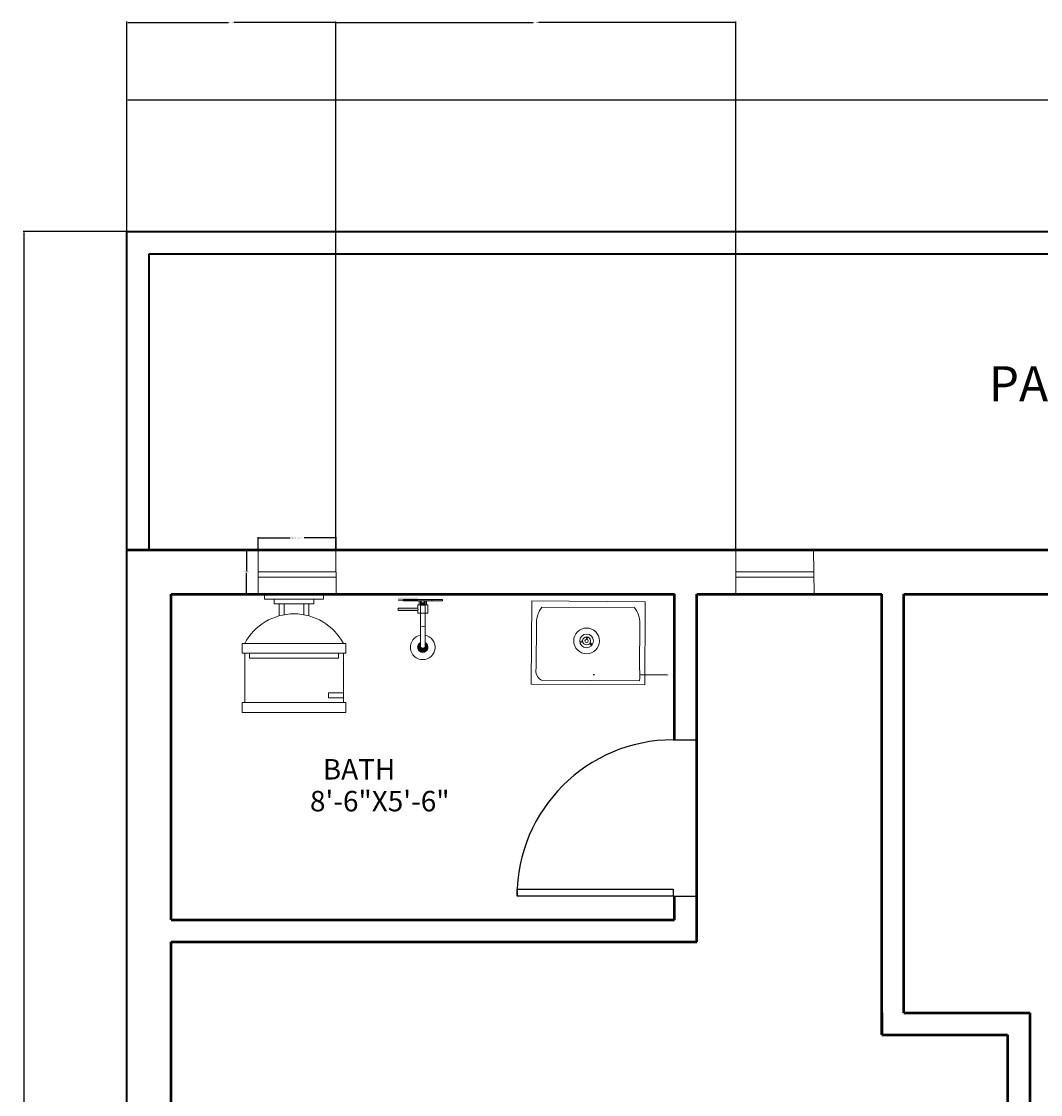
# Model space of a CAD drawing. Units: inches. Extents: x -44 to 461, y -6 to 860.
# Tile 3 of 7: x -23 to 184, y 642 to 860. Entities that reach past the tile are written whole.
import ezdxf

# ---------------------------------------------------------------- set-up
doc = ezdxf.new("R2010")
doc.units = ezdxf.units.IN
doc.header["$MEASUREMENT"] = 0
for name, color, linetype, lineweight in [('A-ANNO-DIMS', 2, 'Continuous', 18), ('A-AREA-IDEN', 7, 'Continuous', 18), ('A-DOOR', 4, 'Continuous', 25), ('C-PROP', 7, 'Continuous', 35), ('PLUMBING FIXTURES', 8, 'Continuous', 18), ('walls', 8, 'Continuous', 50), ('windows', 171, 'Continuous', 18)]:
    doc.layers.add(name, color=color, linetype=linetype, lineweight=lineweight)
doc.styles.get("Standard").update_dxf_attribs({"font": 'arial.ttf'})
doc.dimstyles.get("Standard").update_dxf_attribs({"dimtxt": 0.18, "dimasz": 0.18, "dimexe": 0.18, "dimexo": 0.0625, "dimgap": 0.09, "dimtad": 0, "dimtih": 1, "dimtoh": 1, "dimdec": 4, "dimzin": 0, "dimdsep": 46, "dimtxsty": 'Standard', "dimcen": 0.09, "dimadec": 0, "dimazin": 0, "dimtfac": 1, "dimtdec": 4, "dimtofl": 0, "dimtmove": 0, "dimatfit": 3, "dimfxl": 1, "dimtolj": 1, "dimtzin": 0, "dimarcsym": 0})

# ---------------------------------------------------------------- blocks, each defined once
blk = doc.blocks.new('*U10')
for p, q in [((-10, 22), (-10, 12)), ((10, 12), (10, 22)), ((-10, 21), (-7, 21)), ((-7, 20), (-10, 20)), ((-7, 21), (-7, 20)), ((10.5, 12), (-10.5, 12)), ((-10.5, 10), (-10.5, 12)), ((9, 13), (-9, 13)), ((-9, 13), (-9, 12)), ((9, 12), (9, 13)), ((10.5, 12), (10.5, 10)), ((10.5, 10), (-10.5, 10)), ((-3, 4.4065), (-3, 2)), ((3, 2), (3, 4.4065)), ((-2, 2), (-2, 4.1658)), ((2, 4.1658), (2, 2)), ((4, 2), (-4, 2)), ((-4, 2), (-4, 1)), ((4, 1), (4, 2))]:
    blk.add_line(p, q)
for points in [[(10.5, 22), (10.5, 24), (-10.5, 24), (-10.5, 22)], [(6, 0), (6, 1), (-6, 1), (-6, 0)]]:
    blk.add_lwpolyline(points, close=True)
blk.add_arc((0, 15.3333), 11.3333, 208.0725, 331.9275)
blk = doc.blocks.new('*U12')
for p, q in [((0, 0), (0, -6)), ((40, 0), (40, -6))]:
    blk.add_line(p, q)
blk.add_lwpolyline([(0, 0), (0, 40), (1.75, 40), (1.75, 0)], close=True)
blk.add_arc((0, 0), 40, 0, 90)
blk = doc.blocks.new('*D18')
at = {"layer": 'A-ANNO-DIMS', "color": 0, "lineweight": -2, "transparency": 16777216}
for p, q in [((-1.55, 817.11), (-1.55, 843.94)), ((-1.37, 843.76), (207.84, 843.76)), ((418.27, 843.76), (209.05, 843.76)), ((418.45, 817.11), (418.45, 843.94))]:
    blk.add_line(p, q, dxfattribs=at)
at = {"layer": 'A-ANNO-DIMS', "color": 0, "transparency": 16777216}
for points in [[(-1.37, 843.79), (-1.37, 843.73), (-1.55, 843.76)], [(418.27, 843.79), (418.27, 843.73), (418.45, 843.76)]]:
    blk.add_solid(points, dxfattribs=at)
at = {"layer": 'Defpoints', "color": 0, "transparency": 16777216}
for p in [(418.45, 843.76), (-1.55, 817.05), (418.45, 817.05)]:
    blk.add_point(p, dxfattribs=at)
at = {"layer": 'A-ANNO-DIMS', "color": 0, "transparency": 16777216, "insert": (208.45, 843.76), "char_height": 0.18, "attachment_point": 5}
blk.add_mtext('\\A1;420.0000', dxfattribs=at)
blk = doc.blocks.new('*D19')
at = {"layer": 'A-ANNO-DIMS', "color": 0, "lineweight": -2, "transparency": 16777216}
for p, q in [((-1.62, 817.05), (-22.6, 817.05)), ((-22.42, 816.87), (-22.42, 427.23)), ((-22.42, 37.23), (-22.42, 426.87)), ((-1.62, 37.05), (-22.6, 37.05))]:
    blk.add_line(p, q, dxfattribs=at)
at = {"layer": 'A-ANNO-DIMS', "color": 0, "transparency": 16777216}
for points in [[(-22.45, 816.87), (-22.39, 816.87), (-22.42, 817.05)], [(-22.45, 37.23), (-22.39, 37.23), (-22.42, 37.05)]]:
    blk.add_solid(points, dxfattribs=at)
at = {"layer": 'Defpoints', "color": 0, "transparency": 16777216}
for p in [(-22.42, 817.05), (-1.55, 817.05), (-1.55, 37.05)]:
    blk.add_point(p, dxfattribs=at)
at = {"layer": 'A-ANNO-DIMS', "color": 0, "transparency": 16777216, "insert": (-22.42, 427.05), "char_height": 0.18, "attachment_point": 5}
blk.add_mtext('\\A1;780.0000', dxfattribs=at)
blk = doc.blocks.new('WIN-16IN-FRAME')
for p, q in [((0, 0), (0, 9)), ((0, 9), (15.73, 9)), ((15.73, 9), (15.83, 0)), ((15.78, 4.5), (0, 4.5)), ((0, 0), (0, 3.42)), ((0, 3.42), (15.78, 3.42)), ((0.11, 0), (15.83, 0))]:
    blk.add_line(p, q)
blk = doc.blocks.new('LAV-RECTANGULAR')
for p, q in [((0, 0.15), (0.11, 17)), ((0.11, 17), (23.11, 16.85)), ((20.97, 15.65), (2.16, 15.77)), ((23.1, 15.71), (23, 0)), ((23.11, 16.85), (23.1, 15.71)), ((0.99, 3.35), (1.05, 12.64)), ((21.97, 3.21), (22.03, 12.5)), ((10.4, 8.91), (9.84, 8.81)), ((11.22, 9.73), (11.17, 9.24)), ((11.36, 9.22), (11.4, 9.7)), ((10.52, 8.7), (9.87, 8.58)), ((11.84, 8.39), (12.22, 7.95)), ((11.97, 8.6), (12.36, 8.13)), ((23, 0), (0, 0.15)), ((21.95, 0.84), (2.06, 0.97))]:
    blk.add_line(p, q)
for radius in [2.61, 1.39, 0.816, 0.338]:
    blk.add_circle((11.22, 8.91), radius)
for centre, radius, start, end in [((6.46, 12.5), 5.4, 142.7525, 178.5493), ((16.62, 12.43), 5.4, 0.6949, 36.4918), ((3, 2.82), 2.08, 165.2338, 242.9258), ((12.7, 2.09), 9.33, 352.3124, 6.9318)]:
    blk.add_arc(centre, radius, start, end)
blk = doc.blocks.new('O.H SHOWER-PL')
at = {"layer": 'PLUMBING FIXTURES'}
for points in [[(-1.84, 0), (-1.84, -0.25), (1.84, -0.25), (1.84, 0)], [(0.46, -8.72), (0.46, -9.67, -0.422337), (-0.46, -9.67), (-0.46, -8.72, 4.325472)]]:
    blk.add_hatch(color=256, dxfattribs=at).paths.add_polyline_path(points)
for p, q in [((-1.84, 0), (-1.84, -0.25)), ((1.84, 0), (-1.84, 0)), ((1.84, 0), (1.84, -0.25)), ((1.84, -0.25), (-1.84, -0.25)), ((-0.46, -0.25), (-0.46, -9.67)), ((0.46, -0.25), (0.46, -9.67))]:
    blk.add_line(p, q, dxfattribs=at)
for centre, radius, start, end in [((0, -4.48), 1.03, 243.53, 296.47), ((0, -9.67), 2.5, 100.61, 79.39), ((0, -9.67), 1.05, 116.0349, 63.9652), ((0, -9.22), 0.643, 224.2078, 315.7922)]:
    blk.add_arc(centre, radius, start, end, dxfattribs=at)
blk = doc.blocks.new('DIVERTER-PL')
at = {"layer": 'PLUMBING FIXTURES'}
for points in [[(4, 0), (-4, 0), (-4, -0.25), (4, -0.25)], [(0.38, -1.14), (0.38, -0.7), (-0.37, -0.7), (-0.37, -1.14)], [(1, -1.75, 0.30818), (1, -2.25), (5, -2.25), (5, -1.75)]]:
    blk.add_hatch(color=256, dxfattribs=at).paths.add_polyline_path(points)
for p, q in [((-4, 0), (-4, -0.25)), ((-4, 0), (4, 0)), ((4, 0), (4, -0.25)), ((-4, -0.25), (4, -0.25)), ((-4, -0.25), (4, -0.25)), ((-1, -1.05), (-0.37, -1.05)), ((-1, -1.05), (-1, -2.75)), ((-0.75, -0.25), (-0.75, -1.05)), ((-0.37, -0.7), (0.38, -0.7)), ((-0.37, -0.7), (-0.37, -1.14)), ((-0.37, -1.14), (0.38, -1.14)), ((-0.32, -0.7), (-0.32, -0.25)), ((0.32, -0.7), (0.32, -0.25)), ((0.38, -0.7), (0.38, -1.14)), ((0.38, -1.05), (1, -1.05)), ((0.75, -0.25), (0.75, -1.05)), ((1, -1.05), (1, -1.75)), ((-1, -2.75), (1, -2.75)), ((1, -2.25), (1, -2.75))]:
    blk.add_line(p, q, dxfattribs=at)
at = {"layer": 'PLUMBING FIXTURES', "ltscale": 12}
for p, q in [((1, -1.75), (5, -1.75)), ((5, -2.25), (5, -1.75)), ((1, -2.25), (5, -2.25))]:
    blk.add_line(p, q, dxfattribs=at)
at = {"layer": 'PLUMBING FIXTURES'}
blk.add_arc((1.37, -2), 0.444, 145.7435, 214.2565, dxfattribs=at)
blk = doc.blocks.new('A$C7F153053')
at = {"layer": 'PLUMBING FIXTURES', "xscale": -1, "rotation": 270}
for name in ['DIVERTER-PL', 'O.H SHOWER-PL']:
    blk.add_blockref(name, (12.17, 4), dxfattribs=at)
blk = doc.blocks.new('SHOWER-HEAD-AND-DIVERTER')
for points in [[(4, 12.56, -0.30818), (4, 12.06), (0, 12.06), (0, 12.56)], [(4, 12.56, -0.30818), (4, 12.06), (0, 12.06), (0, 12.56)], [(4, 12.56, -0.30818), (4, 12.06), (0, 12.06), (0, 12.56)], [(4, 12.56, -0.30818), (4, 12.06), (0, 12.06), (0, 12.56)], [(4, 12.56, -0.30818), (4, 12.06), (0, 12.06), (0, 12.56)], [(4, 12.56, -0.30818), (4, 12.06), (0, 12.06), (0, 12.56)], [(4, 12.56, -0.30818), (4, 12.06), (0, 12.06), (0, 12.56)], [(4, 12.56, -0.30818), (4, 12.06), (0, 12.06), (0, 12.56)], [(4, 12.56, -0.30818), (4, 12.06), (0, 12.06), (0, 12.56)], [(4, 12.56, -0.30818), (4, 12.06), (0, 12.06), (0, 12.56)], [(4, 12.56, -0.30818), (4, 12.06), (0, 12.06), (0, 12.56)], [(4, 12.56, -0.30818), (4, 12.06), (0, 12.06), (0, 12.56)], [(4, 12.56, -0.30818), (4, 12.06), (0, 12.06), (0, 12.56)], [(4, 12.56, -0.30818), (4, 12.06), (0, 12.06), (0, 12.56)], [(4, 12.56, -0.30818), (4, 12.06), (0, 12.06), (0, 12.56)], [(4, 12.56, -0.30818), (4, 12.06), (0, 12.06), (0, 12.56)], [(4, 12.56, -0.30818), (4, 12.06), (0, 12.06), (0, 12.56)], [(4, 12.56, -0.30818), (4, 12.06), (0, 12.06), (0, 12.56)], [(4, 12.56, -0.30818), (4, 12.06), (0, 12.06), (0, 12.56)], [(4, 12.56, -0.30818), (4, 12.06), (0, 12.06), (0, 12.56)], [(4, 12.56, -0.30818), (4, 12.06), (0, 12.06), (0, 12.56)], [(4, 12.56, -0.30818), (4, 12.06), (0, 12.06), (0, 12.56)], [(4, 12.56, -0.30818), (4, 12.06), (0, 12.06), (0, 12.56)], [(4, 12.56, -0.30818), (4, 12.06), (0, 12.06), (0, 12.56)], [(4, 12.56, -0.30818), (4, 12.06), (0, 12.06), (0, 12.56)], [(4, 12.56, -0.30818), (4, 12.06), (0, 12.06), (0, 12.56)], [(4, 12.56, -0.30818), (4, 12.06), (0, 12.06), (0, 12.56)], [(4, 12.56, -0.30818), (4, 12.06), (0, 12.06), (0, 12.56)], [(4, 12.56, -0.30818), (4, 12.06), (0, 12.06), (0, 12.56)], [(4, 12.56, -0.30818), (4, 12.06), (0, 12.06), (0, 12.56)], [(4, 12.56, -0.30818), (4, 12.06), (0, 12.06), (0, 12.56)], [(4, 12.56, -0.30818), (4, 12.06), (0, 12.06), (0, 12.56)], [(4, 12.56, -0.30818), (4, 12.06), (0, 12.06), (0, 12.56)], [(4, 12.56, -0.30818), (4, 12.06), (0, 12.06), (0, 12.56)], [(4, 12.56, -0.30818), (4, 12.06), (0, 12.06), (0, 12.56)], [(4, 12.56, -0.30818), (4, 12.06), (0, 12.06), (0, 12.56)], [(4.54, 3.44), (4.54, 2.5, 0.422337), (5.46, 2.5), (5.46, 3.44, -4.325472)], [(4.54, 3.44), (4.54, 2.5, 0.422337), (5.46, 2.5), (5.46, 3.44, -4.325472)], [(4.54, 3.44), (4.54, 2.5, 0.422337), (5.46, 2.5), (5.46, 3.44, -4.325472)], [(4.54, 3.44), (4.54, 2.5, 0.422337), (5.46, 2.5), (5.46, 3.44, -4.325472)], [(4.54, 3.44), (4.54, 2.5, 0.422337), (5.46, 2.5), (5.46, 3.44, -4.325472)], [(4.54, 3.44), (4.54, 2.5, 0.422337), (5.46, 2.5), (5.46, 3.44, -4.325472)], [(4.54, 3.44), (4.54, 2.5, 0.422337), (5.46, 2.5), (5.46, 3.44, -4.325472)], [(4.54, 3.44), (4.54, 2.5, 0.422337), (5.46, 2.5), (5.46, 3.44, -4.325472)], [(4.54, 3.44), (4.54, 2.5, 0.422337), (5.46, 2.5), (5.46, 3.44, -4.325472)], [(4.54, 3.44), (4.54, 2.5, 0.422337), (5.46, 2.5), (5.46, 3.44, -4.325472)], [(4.54, 3.44), (4.54, 2.5, 0.422337), (5.46, 2.5), (5.46, 3.44, -4.325472)], [(4.54, 3.44), (4.54, 2.5, 0.422337), (5.46, 2.5), (5.46, 3.44, -4.325472)], [(4.54, 3.44), (4.54, 2.5, 0.422337), (5.46, 2.5), (5.46, 3.44, -4.325472)], [(4.54, 3.44), (4.54, 2.5, 0.422337), (5.46, 2.5), (5.46, 3.44, -4.325472)], [(4.54, 3.44), (4.54, 2.5, 0.422337), (5.46, 2.5), (5.46, 3.44, -4.325472)], [(4.54, 3.44), (4.54, 2.5, 0.422337), (5.46, 2.5), (5.46, 3.44, -4.325472)], [(4.54, 3.44), (4.54, 2.5, 0.422337), (5.46, 2.5), (5.46, 3.44, -4.325472)], [(4.54, 3.44), (4.54, 2.5, 0.422337), (5.46, 2.5), (5.46, 3.44, -4.325472)], [(4.54, 3.44), (4.54, 2.5, 0.422337), (5.46, 2.5), (5.46, 3.44, -4.325472)], [(4.54, 3.44), (4.54, 2.5, 0.422337), (5.46, 2.5), (5.46, 3.44, -4.325472)], [(4.54, 3.44), (4.54, 2.5, 0.422337), (5.46, 2.5), (5.46, 3.44, -4.325472)], [(4.54, 3.44), (4.54, 2.5, 0.422337), (5.46, 2.5), (5.46, 3.44, -4.325472)], [(4.54, 3.44), (4.54, 2.5, 0.422337), (5.46, 2.5), (5.46, 3.44, -4.325472)], [(4.54, 3.44), (4.54, 2.5, 0.422337), (5.46, 2.5), (5.46, 3.44, -4.325472)], [(4.54, 3.44), (4.54, 2.5, 0.422337), (5.46, 2.5), (5.46, 3.44, -4.325472)], [(4.54, 3.44), (4.54, 2.5, 0.422337), (5.46, 2.5), (5.46, 3.44, -4.325472)], [(4.54, 3.44), (4.54, 2.5, 0.422337), (5.46, 2.5), (5.46, 3.44, -4.325472)], [(4.54, 3.44), (4.54, 2.5, 0.422337), (5.46, 2.5), (5.46, 3.44, -4.325472)], [(4.54, 3.44), (4.54, 2.5, 0.422337), (5.46, 2.5), (5.46, 3.44, -4.325472)], [(4.54, 3.44), (4.54, 2.5, 0.422337), (5.46, 2.5), (5.46, 3.44, -4.325472)], [(4.54, 3.44), (4.54, 2.5, 0.422337), (5.46, 2.5), (5.46, 3.44, -4.325472)], [(4.54, 3.44), (4.54, 2.5, 0.422337), (5.46, 2.5), (5.46, 3.44, -4.325472)], [(4.54, 3.44), (4.54, 2.5, 0.422337), (5.46, 2.5), (5.46, 3.44, -4.325472)], [(4.54, 3.44), (4.54, 2.5, 0.422337), (5.46, 2.5), (5.46, 3.44, -4.325472)], [(4.54, 3.44), (4.54, 2.5, 0.422337), (5.46, 2.5), (5.46, 3.44, -4.325472)], [(4.54, 3.44), (4.54, 2.5, 0.422337), (5.46, 2.5), (5.46, 3.44, -4.325472)], [(4.54, 3.44), (4.54, 2.5, 0.422337), (5.46, 2.5), (5.46, 3.44, -4.325472)], [(4.54, 3.44), (4.54, 2.5, 0.422337), (5.46, 2.5), (5.46, 3.44, -4.325472)]]:
    blk.add_hatch(color=256).paths.add_polyline_path(points)
at = {"ltscale": 12}
blk.add_line((4, 12.06), (0, 12.06), dxfattribs=at)
blk.add_line((4, 12.06), (0, 12.06), dxfattribs=at)
blk.add_line((4, 12.06), (0, 12.06), dxfattribs=at)
blk.add_line((4, 12.06), (0, 12.06), dxfattribs=at)
blk.add_line((4, 12.06), (0, 12.06), dxfattribs=at)
blk.add_line((4, 12.06), (0, 12.06), dxfattribs=at)
blk.add_line((4, 12.06), (0, 12.06), dxfattribs=at)
blk.add_line((4, 12.06), (0, 12.06), dxfattribs=at)
blk.add_line((4, 12.06), (0, 12.06), dxfattribs=at)
blk.add_line((4, 12.06), (0, 12.06), dxfattribs=at)
blk.add_line((4, 12.06), (0, 12.06), dxfattribs=at)
blk.add_line((4, 12.06), (0, 12.06), dxfattribs=at)
blk.add_line((4, 12.06), (0, 12.06), dxfattribs=at)
blk.add_line((4, 12.06), (0, 12.06), dxfattribs=at)
blk.add_line((4, 12.06), (0, 12.06), dxfattribs=at)
blk.add_line((4, 12.06), (0, 12.06), dxfattribs=at)
blk.add_line((4, 12.06), (0, 12.06), dxfattribs=at)
blk.add_line((4, 12.06), (0, 12.06), dxfattribs=at)
blk.add_line((4, 12.06), (0, 12.06), dxfattribs=at)
blk.add_line((4, 12.06), (0, 12.06), dxfattribs=at)
blk.add_line((4, 12.06), (0, 12.06), dxfattribs=at)
blk.add_line((4, 12.06), (0, 12.06), dxfattribs=at)
blk.add_line((4, 12.06), (0, 12.06), dxfattribs=at)
blk.add_line((4, 12.06), (0, 12.06), dxfattribs=at)
blk.add_line((4, 12.06), (0, 12.06), dxfattribs=at)
blk.add_line((4, 12.06), (0, 12.06), dxfattribs=at)
blk.add_line((4, 12.06), (0, 12.06), dxfattribs=at)
blk.add_line((4, 12.06), (0, 12.06), dxfattribs=at)
blk.add_line((4, 12.06), (0, 12.06), dxfattribs=at)
blk.add_line((4, 12.06), (0, 12.06), dxfattribs=at)
blk.add_line((4, 12.06), (0, 12.06), dxfattribs=at)
blk.add_line((4, 12.06), (0, 12.06), dxfattribs=at)
blk.add_line((4, 12.06), (0, 12.06), dxfattribs=at)
blk.add_line((4, 12.06), (0, 12.06), dxfattribs=at)
blk.add_line((4, 12.06), (0, 12.06), dxfattribs=at)
blk.add_line((4, 12.06), (0, 12.06), dxfattribs=at)
blk.add_line((4, 12.06), (0, 12.06), dxfattribs=at)
blk.add_line((4, 12.06), (0, 12.06), dxfattribs=at)
for p, q in [((4.54, 11.92), (4.54, 2.5)), ((4.54, 11.92), (4.54, 2.5)), ((4.54, 11.92), (4.54, 2.5)), ((4.54, 11.92), (4.54, 2.5)), ((4.54, 11.92), (4.54, 2.5)), ((4.54, 11.92), (4.54, 2.5)), ((4.54, 11.92), (4.54, 2.5)), ((4.54, 11.92), (4.54, 2.5)), ((4.54, 11.92), (4.54, 2.5)), ((4.54, 11.92), (4.54, 2.5)), ((4.54, 11.92), (4.54, 2.5)), ((4.54, 11.92), (4.54, 2.5)), ((4.54, 11.92), (4.54, 2.5)), ((4.54, 11.92), (4.54, 2.5)), ((4.54, 11.92), (4.54, 2.5)), ((4.54, 11.92), (4.54, 2.5)), ((4.54, 11.92), (4.54, 2.5)), ((4.54, 11.92), (4.54, 2.5)), ((4.54, 11.92), (4.54, 2.5)), ((4.54, 11.92), (4.54, 2.5)), ((4.54, 11.92), (4.54, 2.5)), ((4.54, 11.92), (4.54, 2.5)), ((4.54, 11.92), (4.54, 2.5)), ((4.54, 11.92), (4.54, 2.5)), ((4.54, 11.92), (4.54, 2.5)), ((4.54, 11.92), (4.54, 2.5)), ((4.54, 11.92), (4.54, 2.5)), ((4.54, 11.92), (4.54, 2.5)), ((4.54, 11.92), (4.54, 2.5)), ((4.54, 11.92), (4.54, 2.5)), ((4.54, 11.92), (4.54, 2.5)), ((4.54, 11.92), (4.54, 2.5)), ((4.54, 11.92), (4.54, 2.5)), ((4.54, 11.92), (4.54, 2.5)), ((4.54, 11.92), (4.54, 2.5)), ((4.54, 11.92), (4.54, 2.5)), ((4.54, 11.92), (4.54, 2.5)), ((4.54, 11.92), (4.54, 2.5)), ((5.46, 11.92), (5.46, 2.5)), ((5.46, 11.92), (5.46, 2.5)), ((5.46, 11.92), (5.46, 2.5)), ((5.46, 11.92), (5.46, 2.5)), ((5.46, 11.92), (5.46, 2.5)), ((5.46, 11.92), (5.46, 2.5)), ((5.46, 11.92), (5.46, 2.5)), ((5.46, 11.92), (5.46, 2.5)), ((5.46, 11.92), (5.46, 2.5)), ((5.46, 11.92), (5.46, 2.5)), ((5.46, 11.92), (5.46, 2.5)), ((5.46, 11.92), (5.46, 2.5)), ((5.46, 11.92), (5.46, 2.5)), ((5.46, 11.92), (5.46, 2.5)), ((5.46, 11.92), (5.46, 2.5)), ((5.46, 11.92), (5.46, 2.5)), ((5.46, 11.92), (5.46, 2.5)), ((5.46, 11.92), (5.46, 2.5)), ((5.46, 11.92), (5.46, 2.5)), ((5.46, 11.92), (5.46, 2.5)), ((5.46, 11.92), (5.46, 2.5)), ((5.46, 11.92), (5.46, 2.5)), ((5.46, 11.92), (5.46, 2.5)), ((5.46, 11.92), (5.46, 2.5)), ((5.46, 11.92), (5.46, 2.5)), ((5.46, 11.92), (5.46, 2.5)), ((5.46, 11.92), (5.46, 2.5)), ((5.46, 11.92), (5.46, 2.5)), ((5.46, 11.92), (5.46, 2.5)), ((5.46, 11.92), (5.46, 2.5)), ((5.46, 11.92), (5.46, 2.5)), ((5.46, 11.92), (5.46, 2.5)), ((5.46, 11.92), (5.46, 2.5)), ((5.46, 11.92), (5.46, 2.5)), ((5.46, 11.92), (5.46, 2.5)), ((5.46, 11.92), (5.46, 2.5)), ((5.46, 11.92), (5.46, 2.5)), ((5.46, 11.92), (5.46, 2.5))]:
    blk.add_line(p, q)
for centre, radius, start, end in [((5, 7.69), 1.03, 243.53, 296.47), ((5, 7.69), 1.03, 243.53, 296.47), ((5, 7.69), 1.03, 243.53, 296.47), ((5, 7.69), 1.03, 243.53, 296.47), ((5, 7.69), 1.03, 243.53, 296.47), ((5, 7.69), 1.03, 243.53, 296.47), ((5, 7.69), 1.03, 243.53, 296.47), ((5, 7.69), 1.03, 243.53, 296.47), ((5, 7.69), 1.03, 243.53, 296.47), ((5, 7.69), 1.03, 243.53, 296.47), ((5, 7.69), 1.03, 243.53, 296.47), ((5, 7.69), 1.03, 243.53, 296.47), ((5, 7.69), 1.03, 243.53, 296.47), ((5, 7.69), 1.03, 243.53, 296.47), ((5, 7.69), 1.03, 243.53, 296.47), ((5, 7.69), 1.03, 243.53, 296.47), ((5, 7.69), 1.03, 243.53, 296.47), ((5, 7.69), 1.03, 243.53, 296.47), ((5, 7.69), 1.03, 243.53, 296.47), ((5, 7.69), 1.03, 243.53, 296.47), ((5, 7.69), 1.03, 243.53, 296.47), ((5, 7.69), 1.03, 243.53, 296.47), ((5, 7.69), 1.03, 243.53, 296.47), ((5, 7.69), 1.03, 243.53, 296.47), ((5, 7.69), 1.03, 243.53, 296.47), ((5, 7.69), 1.03, 243.53, 296.47), ((5, 7.69), 1.03, 243.53, 296.47), ((5, 7.69), 1.03, 243.53, 296.47), ((5, 7.69), 1.03, 243.53, 296.47), ((5, 7.69), 1.03, 243.53, 296.47), ((5, 7.69), 1.03, 243.53, 296.47), ((5, 7.69), 1.03, 243.53, 296.47), ((5, 7.69), 1.03, 243.53, 296.47), ((5, 7.69), 1.03, 243.53, 296.47), ((5, 7.69), 1.03, 243.53, 296.47), ((5, 7.69), 1.03, 243.53, 296.47), ((5, 7.69), 1.03, 243.53, 296.47), ((5, 7.69), 1.03, 243.53, 296.47), ((5, 2.5), 2.5, 100.61, 79.39), ((5, 2.5), 2.5, 100.61, 79.39), ((5, 2.5), 2.5, 100.61, 79.39), ((5, 2.5), 2.5, 100.61, 79.39), ((5, 2.5), 2.5, 100.61, 79.39), ((5, 2.5), 2.5, 100.61, 79.39), ((5, 2.5), 2.5, 100.61, 79.39), ((5, 2.5), 2.5, 100.61, 79.39), ((5, 2.5), 2.5, 100.61, 79.39), ((5, 2.5), 2.5, 100.61, 79.39), ((5, 2.5), 2.5, 100.61, 79.39), ((5, 2.5), 2.5, 100.61, 79.39), ((5, 2.5), 2.5, 100.61, 79.39), ((5, 2.5), 2.5, 100.61, 79.39), ((5, 2.5), 2.5, 100.61, 79.39), ((5, 2.5), 2.5, 100.61, 79.39), ((5, 2.5), 2.5, 100.61, 79.39), ((5, 2.5), 2.5, 100.61, 79.39), ((5, 2.5), 2.5, 100.61, 79.39), ((5, 2.5), 2.5, 100.61, 79.39), ((5, 2.5), 2.5, 100.61, 79.39), ((5, 2.5), 2.5, 100.61, 79.39), ((5, 2.5), 2.5, 100.61, 79.39), ((5, 2.5), 2.5, 100.61, 79.39), ((5, 2.5), 2.5, 100.61, 79.39), ((5, 2.5), 2.5, 100.61, 79.39), ((5, 2.5), 2.5, 100.61, 79.39), ((5, 2.5), 2.5, 100.61, 79.39), ((5, 2.5), 2.5, 100.61, 79.39), ((5, 2.5), 2.5, 100.61, 79.39), ((5, 2.5), 2.5, 100.61, 79.39), ((5, 2.5), 2.5, 100.61, 79.39), ((5, 2.5), 2.5, 100.61, 79.39), ((5, 2.5), 2.5, 100.61, 79.39), ((5, 2.5), 2.5, 100.61, 79.39), ((5, 2.5), 2.5, 100.61, 79.39), ((5, 2.5), 2.5, 100.61, 79.39), ((5, 2.5), 2.5, 100.61, 79.39), ((5, 2.5), 1.05, 116.0348, 63.9651), ((5, 2.5), 1.05, 116.0348, 63.9651), ((5, 2.5), 1.05, 116.0348, 63.9651), ((5, 2.5), 1.05, 116.0348, 63.9651), ((5, 2.5), 1.05, 116.0348, 63.9651), ((5, 2.5), 1.05, 116.0348, 63.9651), ((5, 2.5), 1.05, 116.0348, 63.9651), ((5, 2.5), 1.05, 116.0348, 63.9651), ((5, 2.5), 1.05, 116.0348, 63.9651), ((5, 2.5), 1.05, 116.0348, 63.9651), ((5, 2.5), 1.05, 116.0348, 63.9651), ((5, 2.5), 1.05, 116.0348, 63.9651), ((5, 2.5), 1.05, 116.0348, 63.9651), ((5, 2.5), 1.05, 116.0348, 63.9651), ((5, 2.5), 1.05, 116.0348, 63.9651), ((5, 2.5), 1.05, 116.0348, 63.9651), ((5, 2.5), 1.05, 116.0348, 63.9651), ((5, 2.5), 1.05, 116.0348, 63.9651), ((5, 2.5), 1.05, 116.0348, 63.9651), ((5, 2.5), 1.05, 116.0348, 63.9651), ((5, 2.5), 1.05, 116.0348, 63.9651), ((5, 2.5), 1.05, 116.0348, 63.9651), ((5, 2.5), 1.05, 116.0348, 63.9651), ((5, 2.5), 1.05, 116.0348, 63.9651), ((5, 2.5), 1.05, 116.0348, 63.9651), ((5, 2.5), 1.05, 116.0348, 63.9651), ((5, 2.5), 1.05, 116.0348, 63.9651), ((5, 2.5), 1.05, 116.0348, 63.9651), ((5, 2.5), 1.05, 116.0348, 63.9651), ((5, 2.5), 1.05, 116.0348, 63.9651), ((5, 2.5), 1.05, 116.0348, 63.9651), ((5, 2.5), 1.05, 116.0348, 63.9651), ((5, 2.5), 1.05, 116.0348, 63.9651), ((5, 2.5), 1.05, 116.0348, 63.9651), ((5, 2.5), 1.05, 116.0348, 63.9651), ((5, 2.5), 1.05, 116.0348, 63.9651), ((5, 2.5), 1.05, 116.0348, 63.9651), ((5, 2.5), 1.05, 116.0348, 63.9651), ((5, 2.95), 0.643, 224.2078, 315.7922), ((5, 2.95), 0.643, 224.2078, 315.7922), ((5, 2.95), 0.643, 224.2078, 315.7922), ((5, 2.95), 0.643, 224.2078, 315.7922), ((5, 2.95), 0.643, 224.2078, 315.7922), ((5, 2.95), 0.643, 224.2078, 315.7922), ((5, 2.95), 0.643, 224.2078, 315.7922), ((5, 2.95), 0.643, 224.2078, 315.7922), ((5, 2.95), 0.643, 224.2078, 315.7922), ((5, 2.95), 0.643, 224.2078, 315.7922), ((5, 2.95), 0.643, 224.2078, 315.7922), ((5, 2.95), 0.643, 224.2078, 315.7922), ((5, 2.95), 0.643, 224.2078, 315.7922), ((5, 2.95), 0.643, 224.2078, 315.7922), ((5, 2.95), 0.643, 224.2078, 315.7922), ((5, 2.95), 0.643, 224.2078, 315.7922), ((5, 2.95), 0.643, 224.2078, 315.7922), ((5, 2.95), 0.643, 224.2078, 315.7922), ((5, 2.95), 0.643, 224.2078, 315.7922), ((5, 2.95), 0.643, 224.2078, 315.7922), ((5, 2.95), 0.643, 224.2078, 315.7922), ((5, 2.95), 0.643, 224.2078, 315.7922), ((5, 2.95), 0.643, 224.2078, 315.7922), ((5, 2.95), 0.643, 224.2078, 315.7922), ((5, 2.95), 0.643, 224.2078, 315.7922), ((5, 2.95), 0.643, 224.2078, 315.7922), ((5, 2.95), 0.643, 224.2078, 315.7922), ((5, 2.95), 0.643, 224.2078, 315.7922), ((5, 2.95), 0.643, 224.2078, 315.7922), ((5, 2.95), 0.643, 224.2078, 315.7922), ((5, 2.95), 0.643, 224.2078, 315.7922), ((5, 2.95), 0.643, 224.2078, 315.7922), ((5, 2.95), 0.643, 224.2078, 315.7922), ((5, 2.95), 0.643, 224.2078, 315.7922), ((5, 2.95), 0.643, 224.2078, 315.7922), ((5, 2.95), 0.643, 224.2078, 315.7922), ((5, 2.95), 0.643, 224.2078, 315.7922), ((5, 2.95), 0.643, 224.2078, 315.7922)]:
    blk.add_arc(centre, radius, start, end)
at = {"ltscale": 35, "rotation": 89.99999999999999}
blk.add_blockref('A$C7F153053', (9, 0), dxfattribs=at)
blk = doc.blocks.new('*D28')
at = {"layer": 'A-ANNO-DIMS', "color": 0, "lineweight": -2, "transparency": 16777216}
for p, q in [((25.04, 752.61), (25.04, 755.11)), ((25.22, 754.93), (31.52, 754.93)), ((40.69, 754.93), (34.39, 754.93)), ((40.87, 752.61), (40.87, 755.11))]:
    blk.add_line(p, q, dxfattribs=at)
at = {"layer": 'A-ANNO-DIMS', "color": 0, "transparency": 16777216}
for points in [[(25.22, 754.96), (25.22, 754.9), (25.04, 754.93)], [(40.69, 754.96), (40.69, 754.9), (40.87, 754.93)]]:
    blk.add_solid(points, dxfattribs=at)
at = {"layer": 'Defpoints', "color": 0, "transparency": 16777216}
for p in [(40.87, 754.93), (25.04, 752.55), (40.87, 752.55)]:
    blk.add_point(p, dxfattribs=at)
at = {"layer": 'A-ANNO-DIMS', "color": 0, "transparency": 16777216, "insert": (32.95, 754.93), "char_height": 0.18, "attachment_point": 5}
blk.add_mtext('\\A1;WINDOW 15.8344 TYP.', dxfattribs=at)
blk = doc.blocks.new('*D29')
at = {"layer": 'A-ANNO-DIMS', "color": 0, "lineweight": -2, "transparency": 16777216}
for p, q in [((24.97, 752.55), (22.48, 752.55)), ((22.66, 752.37), (22.66, 748.23)), ((22.66, 743.73), (22.66, 747.87)), ((24.97, 743.55), (22.48, 743.55))]:
    blk.add_line(p, q, dxfattribs=at)
at = {"layer": 'A-ANNO-DIMS', "color": 0, "transparency": 16777216}
for points in [[(22.63, 752.37), (22.69, 752.37), (22.66, 752.55)], [(22.63, 743.73), (22.69, 743.73), (22.66, 743.55)]]:
    blk.add_solid(points, dxfattribs=at)
at = {"layer": 'Defpoints', "color": 0, "transparency": 16777216}
for p in [(22.66, 752.55), (25.04, 752.55), (25.04, 743.55)]:
    blk.add_point(p, dxfattribs=at)
at = {"layer": 'A-ANNO-DIMS', "color": 0, "transparency": 16777216, "insert": (22.66, 748.05), "char_height": 0.18, "attachment_point": 5}
blk.add_mtext('\\A1;9.0000 TYP.', dxfattribs=at)
blk = doc.blocks.new('*D64')
at = {"layer": 'A-ANNO-DIMS', "color": 0, "lineweight": -2, "transparency": 16777216}
for p, q in [((-1.55, 752.61), (-1.55, 859.63)), ((-1.37, 859.45), (19.07, 859.45)), ((40.59, 859.45), (20.14, 859.45)), ((40.77, 752.61), (40.77, 859.63))]:
    blk.add_line(p, q, dxfattribs=at)
at = {"layer": 'A-ANNO-DIMS', "color": 0, "transparency": 16777216}
for points in [[(-1.37, 859.48), (-1.37, 859.42), (-1.55, 859.45)], [(40.59, 859.48), (40.59, 859.42), (40.77, 859.45)]]:
    blk.add_solid(points, dxfattribs=at)
at = {"layer": 'Defpoints', "color": 0, "transparency": 16777216}
for p in [(40.77, 859.45), (-1.55, 752.55), (40.77, 752.55)]:
    blk.add_point(p, dxfattribs=at)
at = {"layer": 'A-ANNO-DIMS', "color": 0, "transparency": 16777216, "insert": (19.61, 859.45), "char_height": 0.18, "attachment_point": 5}
blk.add_mtext('\\A1;42.3210', dxfattribs=at)
blk = doc.blocks.new('*D65')
at = {"layer": 'A-ANNO-DIMS', "color": 0, "lineweight": -2, "transparency": 16777216}
for p, q in [((40.77, 752.61), (40.77, 859.63)), ((40.95, 859.45), (80.8, 859.45)), ((121.71, 859.45), (81.86, 859.45)), ((121.89, 752.61), (121.89, 859.63))]:
    blk.add_line(p, q, dxfattribs=at)
at = {"layer": 'A-ANNO-DIMS', "color": 0, "transparency": 16777216}
for points in [[(40.95, 859.48), (40.95, 859.42), (40.77, 859.45)], [(121.71, 859.48), (121.71, 859.42), (121.89, 859.45)]]:
    blk.add_solid(points, dxfattribs=at)
at = {"layer": 'Defpoints', "color": 0, "transparency": 16777216}
for p in [(121.89, 859.45), (40.77, 752.55), (121.89, 752.55)]:
    blk.add_point(p, dxfattribs=at)
at = {"layer": 'A-ANNO-DIMS', "color": 0, "transparency": 16777216, "insert": (81.33, 859.45), "char_height": 0.18, "attachment_point": 5}
blk.add_mtext('\\A1;81.1266', dxfattribs=at)
blk = doc.blocks.new('*D70')
at = {"layer": 'A-ANNO-DIMS', "color": 0, "lineweight": -2, "transparency": 16777216}
for p, q in [((93.02, 727.24), (93.2, 727.24)), ((93.11, 727.15), (93.11, 727.33)), ((108.04, 727.15), (102.62, 727.18))]:
    blk.add_line(p, q, dxfattribs=at)
at = {"layer": 'A-ANNO-DIMS', "color": 0, "transparency": 16777216}
blk.add_solid([(102.62, 727.21), (102.62, 727.15), (102.44, 727.18)], dxfattribs=at)
at = {"layer": 'Defpoints', "color": 0, "transparency": 16777216}
for p in [(93.11, 727.24), (102.44, 727.18)]:
    blk.add_point(p, dxfattribs=at)
at = {"layer": 'A-ANNO-DIMS', "color": 0, "transparency": 16777216, "insert": (108.78, 727.15), "char_height": 0.18, "attachment_point": 5}
blk.add_mtext('\\A1;2X R9.3297', dxfattribs=at)

msp = doc.modelspace()

# ---------------------------------------------------------------- linework, layer by layer
at = {"layer": 'C-PROP'}
for p, q in [((-1.55432, 817.0501), (418.44568, 817.0501)), ((-1.55432, 37.0501), (-1.55432, 817.0501)), ((2.94568, 812.5501), (413.94568, 812.5501)), ((2.94568, 752.5501), (2.94568, 812.5501)), ((-1.55432, 752.5501), (2.94568, 752.5501))]:
    msp.add_line(p, q, dxfattribs=at)
at = {"layer": 'walls'}
for p, q in [((-1.55432, 752.5501), (358.44568, 752.5501)), ((7.44568, 743.5501), (109.44568, 743.5501)), ((7.44568, 677.5501), (7.44568, 743.5501)), ((109.44568, 714.00861), (109.44568, 743.5501)), ((113.94568, 743.5501), (151.44568, 743.5501)), ((113.94568, 673.0501), (113.94568, 743.5501)), ((151.44568, 654.18945), (151.44568, 743.5501)), ((155.94568, 743.5501), (349.44568, 743.5501)), ((155.94568, 658.68945), (155.94568, 743.5501)), ((109.44568, 677.5501), (109.44568, 682.34129)), ((7.44568, 677.5501), (109.44568, 677.5501)), ((7.44568, 673.0501), (113.94568, 673.0501)), ((7.44568, 505.0501), (7.44568, 673.0501)), ((151.44568, 658.68945), (151.44568, 654.18945)), ((155.94568, 658.68945), (181.44568, 658.68945)), ((181.44568, 658.68945), (181.44568, 610.0501)), ((151.44568, 654.18945), (176.94568, 654.18945)), ((176.94568, 654.18945), (176.94568, 605.5501))]:
    msp.add_line(p, q, dxfattribs=at)

# ---------------------------------------------------------------- block references
at = {"layer": 'A-DOOR', "xscale": 0.7916830879858355, "yscale": 0.7916830879858355, "zscale": 0.7916830879858355, "rotation": 90}
msp.add_blockref('*U12', (109.19559, 682.34129), dxfattribs=at)
at = {"layer": 'PLUMBING FIXTURES', "rotation": 180}
msp.add_blockref('*U10', (32.32147, 743.5501), dxfattribs=at)
at = {"layer": 'PLUMBING FIXTURES'}
for name, p in [('SHOWER-HEAD-AND-DIVERTER', (53.414, 730.279)), ('LAV-RECTANGULAR', (80.406, 725.157))]:
    msp.add_blockref(name, p, dxfattribs=at)
at = {"layer": 'windows'}
for p in [(25.037, 743.55), (121.89311, 743.55)]:
    msp.add_blockref('WIN-16IN-FRAME', p, dxfattribs=at)

# ---------------------------------------------------------------- texts
at = {"layer": 'A-AREA-IDEN'}
for s, height, p in [('PASSAGE 5\'-4.5" WIDE', 7.1129656, (173.13701, 782.63673)), ('BATH', 4.155577, (38.1506, 705.96146)), ('8\'-6"X5\'-6"', 4.1555773, (35.55054, 699.50357))]:
    msp.add_text(s, height=height, dxfattribs=at).set_placement(p)

# ---------------------------------------------------------------- dimensions: what is measured, and where the dimension line sits
at = {"layer": 'A-ANNO-DIMS'}
for base, p1, p2, override, picture, middle in [((40.76669, 859.4501), (-1.55431, 752.5501), (40.76669, 752.5501), {"dimdec": 4, "dimlfac": 1, "dimrnd": 0, "dimzin": 0, "dimdsep": 46, "dimlunit": 2}, '*D64', (19.60619, 859.4501)), ((121.89333, 859.4501), (40.76669, 752.5501), (121.89333, 752.5501), {"dimdec": 4, "dimlfac": 1, "dimrnd": 0, "dimzin": 0, "dimdsep": 46, "dimlunit": 2}, '*D65', (81.33001, 859.4501)), ((418.44568, 843.76223), (-1.55432, 817.0501), (418.44568, 817.0501), {"dimclrd": 0, "dimclre": 0, "dimclrt": 0}, '*D18', (208.44568, 843.76223))]:
    dim = msp.add_linear_dim(base=base, p1=p1, p2=p2, dimstyle='Standard', override=override, dxfattribs=at)
    dim.commit()
    dim.dimension.update_dxf_attribs({"geometry": picture, "text_midpoint": middle})
dim = msp.add_linear_dim(base=(-22.41551, 817.0501), p1=(-1.55432, 37.0501), p2=(-1.55432, 817.0501), angle=90, dimstyle='Standard', override={"dimclrd": 0, "dimclre": 0, "dimclrt": 0}, dxfattribs=at)
dim.commit()
dim.dimension.update_dxf_attribs({"geometry": '*D19', "text_midpoint": (-22.41551, 427.0501)})
dim = msp.add_linear_dim(base=(40.87165, 754.92526), p1=(25.03722, 752.5501), p2=(40.87165, 752.5501), text='WINDOW <> TYP.', dimstyle='Standard', override={"dimdec": 4, "dimlfac": 1, "dimrnd": 0, "dimzin": 0, "dimdsep": 46, "dimlunit": 2}, dxfattribs=at)
dim.commit()
dim.dimension.update_dxf_attribs({"geometry": '*D28', "text_midpoint": (32.95443, 754.92526)})
dim = msp.add_linear_dim(base=(22.66205, 752.5501), p1=(25.03722, 743.5501), p2=(25.03722, 752.5501), angle=90, text='<> TYP.', dimstyle='Standard', override={"dimdec": 4, "dimlfac": 1, "dimrnd": 0, "dimzin": 0, "dimdsep": 46, "dimlunit": 2}, dxfattribs=at)
dim.commit()
dim.dimension.update_dxf_attribs({"geometry": '*D29', "text_midpoint": (22.66205, 748.0501)})
dim = msp.add_radius_dim(center=(93.11023, 727.24478), mpoint=(102.43977, 727.183), text='2X <>', dimstyle='Standard', override={"dimdec": 4, "dimlfac": 1, "dimrnd": 0, "dimzin": 0, "dimdsep": 46, "dimlunit": 2}, dxfattribs=at)
dim.commit()
dim.dimension.update_dxf_attribs({"geometry": '*D70', "text_midpoint": (108.0375, 727.14594), "dimtype": 164})

doc.saveas('drawing.dxf')
